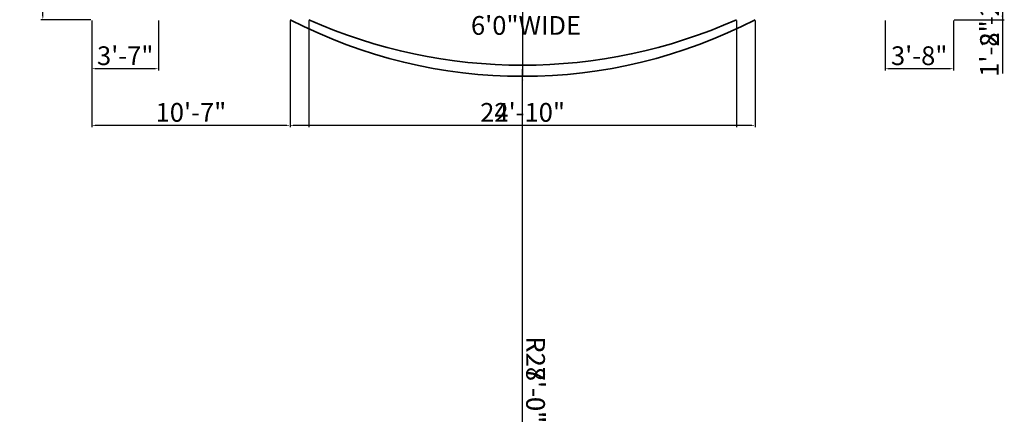
# Model space of a CAD drawing. Units: inches. Extents: x 1749 to 2426, y 1666 to 2412.
# Tile 1 of 3: x 1776 to 2407, y 1666 to 1924. Entities that reach past the tile are written whole.
import ezdxf

# ---------------------------------------------------------------- set-up
doc = ezdxf.new("R2010")
doc.units = ezdxf.units.IN
for name, color, linetype, lineweight in [('A-ANNO-DIMS', 2, 'Continuous', 18), ('A-AREA-IDEN', 4, 'Continuous', 18), ('A-WALL', 2, 'Continuous', 35)]:
    doc.layers.add(name, color=color, linetype=linetype, lineweight=lineweight)
doc.styles.get("Standard").update_dxf_attribs({"font": 'arial.ttf'})
doc.dimstyles.new('ISO-25', dxfattribs={"dimtxt": 12, "dimasz": 2.5, "dimexe": 1.25, "dimexo": 0.625, "dimtad": 1, "dimdec": 0, "dimlunit": 3, "dimtxsty": 'Standard', "dimcen": 2.5, "dimadec": 0, "dimazin": 0, "dimtfac": 1, "dimtdec": 0, "dimtmove": 0, "dimatfit": 3, "dimfxl": 1, "dimarcsym": 0})

# ---------------------------------------------------------------- blocks, each defined once
blk = doc.blocks.new('*D26')
at = {"layer": 'A-ANNO-DIMS', "color": 0, "lineweight": -2, "transparency": 16777216}
for p, q in [((1822.59, 1923.6), (1822.59, 1855.28)), ((1949.59, 1923.6), (1949.59, 1855.28)), ((1825.09, 1856.53), (1947.09, 1856.53))]:
    blk.add_line(p, q, dxfattribs=at)
at = {"layer": 'A-ANNO-DIMS', "color": 0, "transparency": 16777216}
for points in [[(1825.09, 1856.94), (1825.09, 1856.11), (1822.59, 1856.53)], [(1947.09, 1856.94), (1947.09, 1856.11), (1949.59, 1856.53)]]:
    blk.add_solid(points, dxfattribs=at)
at = {"layer": 'Defpoints', "color": 0, "transparency": 16777216}
for p in [(1822.59, 1924.22), (1949.59, 1924.22), (1949.59, 1856.53)]:
    blk.add_point(p, dxfattribs=at)
at = {"layer": 'A-ANNO-DIMS', "color": 0, "transparency": 16777216, "insert": (1886.09, 1863.28), "char_height": 12, "attachment_point": 5}
blk.add_mtext('10\'-7"', dxfattribs=at)
blk = doc.blocks.new('*D27')
at = {"layer": 'A-ANNO-DIMS', "color": 0, "lineweight": -2, "transparency": 16777216}
for p, q in [((1949.59, 1923.6), (1949.59, 1855.28)), ((2247.59, 1923.6), (2247.59, 1855.28)), ((1952.09, 1856.53), (2245.09, 1856.53))]:
    blk.add_line(p, q, dxfattribs=at)
at = {"layer": 'A-ANNO-DIMS', "color": 0, "transparency": 16777216}
for points in [[(1952.09, 1856.94), (1952.09, 1856.11), (1949.59, 1856.53)], [(2245.09, 1856.94), (2245.09, 1856.11), (2247.59, 1856.53)]]:
    blk.add_solid(points, dxfattribs=at)
at = {"layer": 'Defpoints', "color": 0, "transparency": 16777216}
for p in [(1949.59, 1924.22), (2247.59, 1924.22), (2247.59, 1856.53)]:
    blk.add_point(p, dxfattribs=at)
at = {"layer": 'A-ANNO-DIMS', "color": 0, "transparency": 16777216, "insert": (2098.59, 1863.28), "char_height": 12, "attachment_point": 5}
blk.add_mtext('24\'-10"', dxfattribs=at)
blk = doc.blocks.new('*D28')
at = {"layer": 'A-ANNO-DIMS', "color": 0, "lineweight": -2, "transparency": 16777216}
for p, q in [((1961.59, 1923.6), (1961.59, 1855.28)), ((2235.59, 1923.6), (2235.59, 1855.28)), ((1964.09, 1856.53), (2233.09, 1856.53))]:
    blk.add_line(p, q, dxfattribs=at)
at = {"layer": 'A-ANNO-DIMS', "color": 0, "transparency": 16777216}
for points in [[(1964.09, 1856.94), (1964.09, 1856.11), (1961.59, 1856.53)], [(2233.09, 1856.94), (2233.09, 1856.11), (2235.59, 1856.53)]]:
    blk.add_solid(points, dxfattribs=at)
at = {"layer": 'Defpoints', "color": 0, "transparency": 16777216}
for p in [(1961.59, 1924.22), (2235.59, 1924.22), (2235.59, 1856.53)]:
    blk.add_point(p, dxfattribs=at)
at = {"layer": 'A-ANNO-DIMS', "color": 0, "transparency": 16777216, "insert": (2098.59, 1863.28), "char_height": 12, "attachment_point": 5}
blk.add_mtext('22\'-10"', dxfattribs=at)
blk = doc.blocks.new('*D41')
at = {"layer": 'A-ANNO-DIMS', "color": 0, "lineweight": -2, "transparency": 16777216}
for p, q in [((1791.19, 1940.27), (1791.19, 1974.79)), ((1821.97, 1940.27), (1789.94, 1940.27)), ((1791.19, 1926.72), (1791.19, 1937.77)), ((1821.97, 1924.22), (1789.94, 1924.22))]:
    blk.add_line(p, q, dxfattribs=at)
at = {"layer": 'A-ANNO-DIMS', "color": 0, "transparency": 16777216}
for points in [[(1790.77, 1937.77), (1791.61, 1937.77), (1791.19, 1940.27)], [(1790.77, 1926.72), (1791.61, 1926.72), (1791.19, 1924.22)]]:
    blk.add_solid(points, dxfattribs=at)
at = {"layer": 'Defpoints', "color": 0, "transparency": 16777216}
for p in [(1791.19, 1940.27), (1822.59, 1940.27), (1822.59, 1924.22)]:
    blk.add_point(p, dxfattribs=at)
at = {"layer": 'A-ANNO-DIMS', "color": 0, "transparency": 16777216, "insert": (1784.54, 1958.78), "char_height": 12, "attachment_point": 5, "rotation": 90}
blk.add_mtext('1\'-4"', dxfattribs=at)
blk = doc.blocks.new('*D42')
at = {"layer": 'A-ANNO-DIMS', "color": 0, "lineweight": -2, "transparency": 16777216}
for p, q in [((2375.22, 1970.3), (2407.24, 1970.3)), ((2405.99, 1967.8), (2405.99, 1946.8)), ((2375.22, 1944.3), (2407.24, 1944.3)), ((2405.99, 1944.3), (2405.99, 1908.45))]:
    blk.add_line(p, q, dxfattribs=at)
at = {"layer": 'A-ANNO-DIMS', "color": 0, "transparency": 16777216}
for points in [[(2405.57, 1967.8), (2406.41, 1967.8), (2405.99, 1970.3)], [(2405.57, 1946.8), (2406.41, 1946.8), (2405.99, 1944.3)]]:
    blk.add_solid(points, dxfattribs=at)
at = {"layer": 'Defpoints', "color": 0, "transparency": 16777216}
for p in [(2374.59, 1970.3), (2374.59, 1944.3), (2405.99, 1944.3)]:
    blk.add_point(p, dxfattribs=at)
at = {"layer": 'A-ANNO-DIMS', "color": 0, "transparency": 16777216, "insert": (2399.34, 1925.13), "char_height": 12, "attachment_point": 5, "rotation": 90}
blk.add_mtext('2\'-2"', dxfattribs=at)
blk = doc.blocks.new('*D43')
at = {"layer": 'A-ANNO-DIMS', "color": 0, "lineweight": -2, "transparency": 16777216}
for p, q in [((2375.22, 1944.3), (2407.24, 1944.3)), ((2405.99, 1941.8), (2405.99, 1926.72)), ((2375.22, 1924.22), (2407.24, 1924.22)), ((2405.99, 1924.22), (2405.99, 1889.7))]:
    blk.add_line(p, q, dxfattribs=at)
at = {"layer": 'A-ANNO-DIMS', "color": 0, "transparency": 16777216}
for points in [[(2405.57, 1941.8), (2406.41, 1941.8), (2405.99, 1944.3)], [(2405.57, 1926.72), (2406.41, 1926.72), (2405.99, 1924.22)]]:
    blk.add_solid(points, dxfattribs=at)
at = {"layer": 'Defpoints', "color": 0, "transparency": 16777216}
for p in [(2374.59, 1944.3), (2374.59, 1924.22), (2405.99, 1924.22)]:
    blk.add_point(p, dxfattribs=at)
at = {"layer": 'A-ANNO-DIMS', "color": 0, "transparency": 16777216, "insert": (2399.24, 1905.71), "char_height": 12, "attachment_point": 5, "rotation": 90}
blk.add_mtext('1\'-8"', dxfattribs=at)
blk = doc.blocks.new('*D44')
at = {"layer": 'A-ANNO-DIMS', "color": 0, "lineweight": -2, "transparency": 16777216}
for p, q in [((1822.59, 1923.6), (1822.59, 1891.57)), ((1865.37, 1923.6), (1865.37, 1891.57)), ((1862.87, 1892.82), (1825.09, 1892.82))]:
    blk.add_line(p, q, dxfattribs=at)
at = {"layer": 'A-ANNO-DIMS', "color": 0, "transparency": 16777216}
for points in [[(1825.09, 1893.24), (1825.09, 1892.4), (1822.59, 1892.82)], [(1862.87, 1893.24), (1862.87, 1892.4), (1865.37, 1892.82)]]:
    blk.add_solid(points, dxfattribs=at)
at = {"layer": 'Defpoints', "color": 0, "transparency": 16777216}
for p in [(1822.59, 1924.22), (1865.37, 1924.22), (1822.59, 1892.82)]:
    blk.add_point(p, dxfattribs=at)
at = {"layer": 'A-ANNO-DIMS', "color": 0, "transparency": 16777216, "insert": (1843.98, 1899.58), "char_height": 12, "attachment_point": 5}
blk.add_mtext('3\'-7"', dxfattribs=at)
blk = doc.blocks.new('*D45')
at = {"layer": 'A-ANNO-DIMS', "color": 0, "lineweight": -2, "transparency": 16777216}
for p, q in [((2330.81, 1923.6), (2330.81, 1891.57)), ((2374.59, 1923.6), (2374.59, 1891.57)), ((2372.09, 1892.82), (2333.31, 1892.82))]:
    blk.add_line(p, q, dxfattribs=at)
at = {"layer": 'A-ANNO-DIMS', "color": 0, "transparency": 16777216}
for points in [[(2333.31, 1893.24), (2333.31, 1892.4), (2330.81, 1892.82)], [(2372.09, 1893.24), (2372.09, 1892.4), (2374.59, 1892.82)]]:
    blk.add_solid(points, dxfattribs=at)
at = {"layer": 'Defpoints', "color": 0, "transparency": 16777216}
for p in [(2330.81, 1924.22), (2374.59, 1924.22), (2330.81, 1892.82)]:
    blk.add_point(p, dxfattribs=at)
at = {"layer": 'A-ANNO-DIMS', "color": 0, "transparency": 16777216, "insert": (2352.7, 1899.58), "char_height": 12, "attachment_point": 5}
blk.add_mtext('3\'-8"', dxfattribs=at)
blk = doc.blocks.new('*D56')
at = {"layer": 'A-ANNO-DIMS', "color": 0, "lineweight": -2, "transparency": 16777216}
for p, q in [((2098.59, 2231.02), (2098.59, 1895.02)), ((2098.59, 1666.44), (2098.59, 1892.52))]:
    blk.add_line(p, q, dxfattribs=at)
at = {"layer": 'A-ANNO-DIMS', "color": 0, "transparency": 16777216}
blk.add_solid([(2099.01, 1892.52), (2098.18, 1892.52), (2098.59, 1895.02)], dxfattribs=at)
at = {"layer": 'Defpoints', "color": 0, "transparency": 16777216}
for p in [(2098.59, 2231.02), (2098.59, 1895.02)]:
    blk.add_point(p, dxfattribs=at)
at = {"layer": 'A-ANNO-DIMS', "color": 0, "transparency": 16777216, "insert": (2105.34, 1693.42), "char_height": 12, "attachment_point": 5, "rotation": 270.00008}
blk.add_mtext('R28\'-0"', dxfattribs=at)
blk = doc.blocks.new('*D57')
at = {"layer": 'A-ANNO-DIMS', "color": 0, "lineweight": -2, "transparency": 16777216}
for p, q in [((2098.59, 2211.93), (2098.59, 1887.93)), ((2098.59, 1666.55), (2098.59, 1885.43))]:
    blk.add_line(p, q, dxfattribs=at)
at = {"layer": 'A-ANNO-DIMS', "color": 0, "transparency": 16777216}
blk.add_solid([(2099.01, 1885.43), (2098.18, 1885.43), (2098.59, 1887.93)], dxfattribs=at)
at = {"layer": 'Defpoints', "color": 0, "transparency": 16777216}
for p in [(2098.59, 2211.93), (2098.59, 1887.93)]:
    blk.add_point(p, dxfattribs=at)
at = {"layer": 'A-ANNO-DIMS', "color": 0, "transparency": 16777216, "insert": (2105.34, 1693.53), "char_height": 12, "attachment_point": 5, "rotation": 270.00009}
blk.add_mtext('R27\'-0"', dxfattribs=at)

msp = doc.modelspace()

# ---------------------------------------------------------------- linework, layer by layer
at = {"layer": 'A-WALL'}
for centre, radius, start, end in [((2098.59, 2211.93), 324, 242.62086, 297.37914), ((2098.59, 2231.02), 336, 245.93718, 294.06282)]:
    msp.add_arc(centre, radius, start, end, dxfattribs=at)

# ---------------------------------------------------------------- texts
at = {"layer": 'A-AREA-IDEN'}
msp.add_attdef('6\'0"WIDE', (2065.51, 1914.54), '', height=12, dxfattribs=at)

# ---------------------------------------------------------------- dimensions: what is measured, and where the dimension line sits
at = {"layer": 'A-ANNO-DIMS'}
for center, mpoint, picture, middle in [((2098.59, 2231.02), (2098.59, 1895.02), '*D56', (2098.59, 1693.42)), ((2098.59, 2211.93), (2098.59, 1887.93), '*D57', (2098.59, 1693.53))]:
    dim = msp.add_radius_dim(center=center, mpoint=mpoint, dimstyle='ISO-25', override={"dimdec": 1, "dimlfac": 1, "dimrnd": 0, "dimzin": 1, "dimdsep": 46, "dimlunit": 4, "dimfrac": 2}, dxfattribs=at)
    dim.commit()
    dim.dimension.update_dxf_attribs({"geometry": picture, "text_midpoint": middle, "dimtype": 164})
for base, p1, p2, angle, picture, middle in [((1791.1915, 1940.2744), (1822.5915, 1924.2209), (1822.5915, 1940.2744), 90, '*D41', (1784.542, 1958.7842)), ((2405.99, 1944.3), (2374.59, 1970.3), (2374.59, 1944.3), 270, '*D42', (2399.34, 1925.13)), ((2405.99, 1924.22), (2374.59, 1944.3), (2374.59, 1924.22), 270, '*D43', (2399.24, 1905.71)), ((1822.59, 1892.82), (1865.37, 1924.22), (1822.59, 1924.22), 180, '*D44', (1843.98, 1899.58)), ((2330.81, 1892.82), (2374.59, 1924.22), (2330.81, 1924.22), 180, '*D45', (2352.7, 1899.58))]:
    dim = msp.add_linear_dim(base=base, p1=p1, p2=p2, angle=angle, dimstyle='ISO-25', override={"dimdec": 1, "dimlfac": 1, "dimrnd": 0, "dimzin": 1, "dimdsep": 46, "dimlunit": 4, "dimfrac": 2}, dxfattribs=at)
    dim.commit()
    dim.dimension.update_dxf_attribs({"geometry": picture, "text_midpoint": middle})
for base, p1, p2, picture, middle in [((1949.59, 1856.53), (1822.59, 1924.22), (1949.59, 1924.22), '*D26', (1886.09, 1863.28)), ((2247.59, 1856.53), (1949.59, 1924.22), (2247.59, 1924.22), '*D27', (2098.59, 1863.28)), ((2235.59, 1856.53), (1961.59, 1924.22), (2235.59, 1924.22), '*D28', (2098.59, 1863.28))]:
    dim = msp.add_linear_dim(base=base, p1=p1, p2=p2, dimstyle='ISO-25', override={"dimdec": 1, "dimlfac": 1, "dimrnd": 0, "dimzin": 1, "dimdsep": 46, "dimlunit": 4, "dimfrac": 2}, dxfattribs=at)
    dim.commit()
    dim.dimension.update_dxf_attribs({"geometry": picture, "text_midpoint": middle})

doc.saveas('drawing.dxf')
